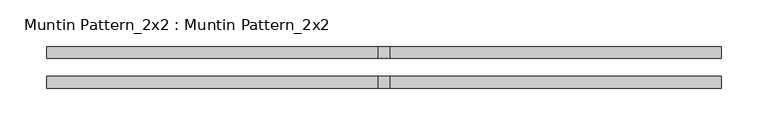
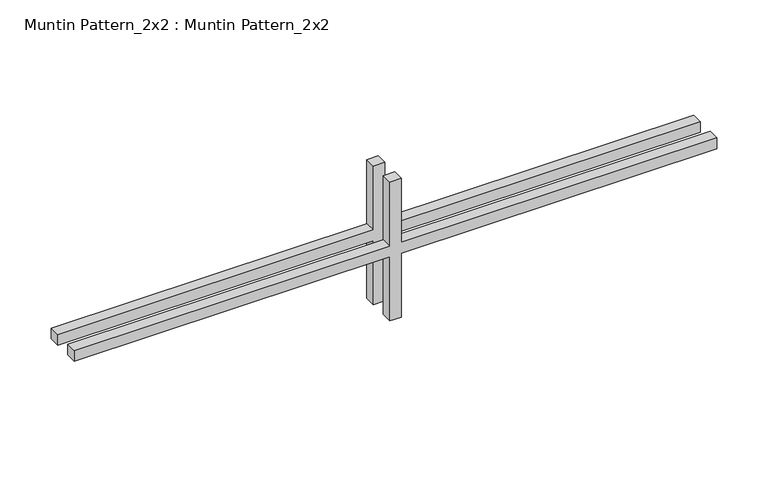
"""IFC4 building model written with IfcOpenShell, lengths in millimetres: proxy geometry, Muntin Pattern_2x2 : Muntin Pattern_2x2."""

from ifc_helpers import new_model, si_unit, frame, origin, place, context, project, spatial, polyline, outline, extrude, source, transform, mapped, element, save


def muntin_pattern_2x2_muntin_pattern_2x2_8320156c(model_context):
    return source(origin(), model_context, "Body", "SweptSolid", [
        extrude(outline(polyline([(88.9, -6.35), (88.9, -361.95), (76.2, -361.95), (76.2, -6.35), (0.0, -6.35), (0.0, 6.35), (76.2, 6.35), (76.2, 361.95), (88.9, 361.95), (88.9, 6.35), (165.1, 6.35), (165.1, -6.35), (88.9, -6.35)])), frame((0.0, -22.225, 0.0), z_axis=(0.0, 1.0, 0.0), x_axis=(0.0, 0.0, 1.0)), (0.0, 0.0, 1.0), 12.7),
        extrude(outline(polyline([(88.9, -6.35), (88.9, -361.95), (76.2, -361.95), (76.2, -6.35), (0.0, -6.35), (0.0, 6.35), (76.2, 6.35), (76.2, 361.95), (88.9, 361.95), (88.9, 6.35), (165.1, 6.35), (165.1, -6.35), (88.9, -6.35)])), frame((0.0, 9.525, 0.0), z_axis=(0.0, 1.0, 0.0), x_axis=(0.0, 0.0, 1.0)), (0.0, 0.0, 1.0), 12.7),
    ])


if __name__ == "__main__":
    model = new_model("IFC4")
    model_context = context("Model", 3, world=origin())
    ifc_project = project(units=[si_unit("LENGTHUNIT", "METRE", prefix="MILLI")], contexts=[model_context])
    site = spatial("IfcSite", under=ifc_project)
    building = spatial("IfcBuilding", under=site)
    placement = place(None, origin())
    muntin_pattern_2x2_muntin_pattern_2x2_shape = muntin_pattern_2x2_muntin_pattern_2x2_8320156c(model_context)
    element("IfcBuildingElementProxy", 1, Name="Muntin Pattern_2x2 : Muntin Pattern_2x2", ObjectType="Muntin Pattern_2x2 : Muntin Pattern_2x2", at=placement, inside=building, context=model_context, shape_type="MappedRepresentation", body=[
        mapped(muntin_pattern_2x2_muntin_pattern_2x2_shape, transform((0.0, 0.0, 0.0), x_axis=(1.0, 0.0, 0.0), y_axis=(0.0, 1.0, 0.0), z_axis=(0.0, 0.0, 1.0))),
    ])
    save(model, "model.ifc")

# Revit data of these elements
# Type "Muntin Pattern_2x2 : Muntin Pattern_2x2"
#   Width [instance default] = 4' - 0"
#   Thickness = 0' - 0 1/2"
#   Height [instance default] = 4' - 0"
#   Distance = 0' - 0 3/4"
#   Interior Material [instance default] = none
#   Exterior Material [instance default] = none
#   Default Elevation = 0
# Element 1 (IfcBuildingElementProxy, "Muntin Pattern_2x2 : Muntin Pattern_2x2")
#   Width = 2' - 4 1/2"
#   Height = 0' - 6 1/2"
#   Interior Material = Wood - Stained
#   Exterior Material = Clad - White
#   Materials on its faces: "Clad - White", "Wood - Stained"
# Materials
#   "Clad - White": class "Wood", colour RGB 242 242 238, transparency 0, Cost = 0
#   "Wood - Stained": class "Wood", colour RGB 224 178 126, transparency 0, Cost = 0
